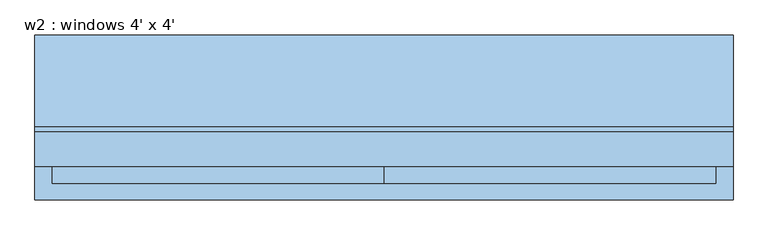
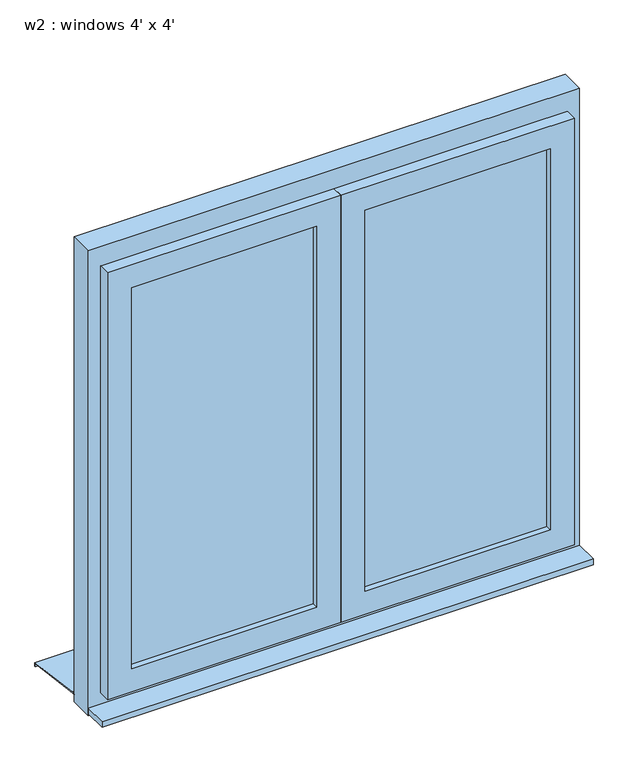
"""IFC4 building model written with IfcOpenShell, lengths in millimetres: window geometry, w2 : windows 4' x 4'."""

from ifc_helpers import new_model, si_unit, frame, origin, place, context, project, spatial, polyline, outline, extrude, faceted_brep, source, transform, mapped, element, save


def w2_windows_4_x_4_9dec5fc7(model_context):
    return source(origin(), model_context, "Body", "SolidModel", [
        extrude(outline(polyline([(-15.6778457, 1020.0), (144.3, 1000.0), (144.3, 990.0), (142.3, 990.0), (142.3, 998.3604634), (-15.8759277, 1018.0), (-25.7, 1018.0), (-25.7, 1020.0), (-15.6778457, 1020.0)])), frame((-609.6, 0.0, 0.0), z_axis=(1.0, 0.0, 0.0), x_axis=(0.0, 1.0, 0.0)), (0.0, 0.0, 1.0), 1219.2),
        extrude(outline(polyline([(-609.6, -144.3), (-609.6, -85.7), (609.6, -85.7), (609.6, -144.3), (-609.6, -144.3)])), frame((0.0, 0.0, 1005.0), z_axis=(0.0, 0.0, 1.0), x_axis=(1.0, 0.0, 0.0)), (0.0, 0.0, 1.0), 15.0),
        extrude(outline(polyline([(60.0, -70.7), (519.6, -70.7), (519.6, -100.7), (60.0, -100.7), (60.0, -70.7)])), frame((0.0, 0.0, 1110.0), z_axis=(0.0, 0.0, 1.0), x_axis=(1.0, 0.0, 0.0)), (0.0, 0.0, 1.0), 999.2),
        extrude(outline(polyline([(-519.6, -70.7), (-60.0, -70.7), (-60.0, -100.7), (-519.6, -100.7), (-519.6, -70.7)])), frame((0.0, 0.0, 1110.0), z_axis=(0.0, 0.0, 1.0), x_axis=(1.0, 0.0, 0.0)), (0.0, 0.0, 1.0), 999.2),
        extrude(outline(polyline([(2219.2, -609.6), (1000.0, -609.6), (1000.0, 609.6), (2219.2, 609.6), (2219.2, -609.6)]), holes=[polyline([(2139.2, -549.6), (2139.2, 549.6), (1080.0, 549.6), (1080.0, -549.6), (2139.2, -549.6)])]), frame((0.0, -85.7, 0.0), z_axis=(0.0, 1.0, 0.0), x_axis=(0.0, 0.0, 1.0)), (0.0, 0.0, 1.0), 60.0),
        extrude(outline(polyline([(30.0, -85.7), (-30.0, -85.7), (-30.0, -25.7), (30.0, -25.7), (30.0, -85.7)])), frame((0.0, 0.0, 1080.0), z_axis=(0.0, 0.0, 1.0), x_axis=(1.0, 0.0, 0.0)), (0.0, 0.0, 1.0), 1059.2),
        faceted_brep([(30.0, -85.7, 1080.0), (30.0, -55.7, 1080.0), (549.6, -55.7, 1080.0), (549.6, -85.7, 1080.0), (549.6, -55.7, 2139.2), (549.6, -85.7, 2139.2), (30.0, -55.7, 2139.2), (519.6, -55.7, 2109.2), (60.0, -55.7, 2109.2), (60.0, -55.7, 1110.0), (519.6, -55.7, 1110.0), (579.6, -85.7, 1050.0), (0.0, -85.7, 1050.0), (0.0, -85.7, 2169.2), (579.6, -85.7, 2169.2), (30.0, -85.7, 2139.2), (0.0, -115.7, 1050.0), (579.6, -115.7, 1050.0), (579.6, -115.7, 2169.2), (0.0, -115.7, 2169.2), (519.6, -115.7, 1110.0), (60.0, -115.7, 1110.0), (60.0, -115.7, 2109.2), (519.6, -115.7, 2109.2)], [[[0, 1, 2, 3]], [[3, 2, 4, 5]], [[2, 1, 6, 4], [7, 8, 9, 10]], [[11, 12, 13, 14], [5, 15, 0, 3]], [[16, 12, 11, 17]], [[17, 11, 14, 18]], [[18, 19, 16, 17], [20, 21, 22, 23]], [[9, 21, 20, 10]], [[10, 20, 23, 7]], [[15, 6, 1, 0]], [[19, 13, 12, 16]], [[8, 22, 21, 9]], [[5, 4, 6, 15]], [[18, 14, 13, 19]], [[7, 23, 22, 8]]]),
        faceted_brep([(-549.6, -85.7, 1080.0), (-549.6, -55.7, 1080.0), (-30.0, -55.7, 1080.0), (-30.0, -85.7, 1080.0), (-30.0, -55.7, 2139.2), (-30.0, -85.7, 2139.2), (-549.6, -55.7, 2139.2), (-60.0, -55.7, 2109.2), (-519.6, -55.7, 2109.2), (-519.6, -55.7, 1110.0), (-60.0, -55.7, 1110.0), (0.0, -85.7, 1050.0), (-579.6, -85.7, 1050.0), (-579.6, -85.7, 2169.2), (0.0, -85.7, 2169.2), (-549.6, -85.7, 2139.2), (-579.6, -115.7, 1050.0), (0.0, -115.7, 1050.0), (0.0, -115.7, 2169.2), (-579.6, -115.7, 2169.2), (-60.0, -115.7, 1110.0), (-519.6, -115.7, 1110.0), (-519.6, -115.7, 2109.2), (-60.0, -115.7, 2109.2)], [[[0, 1, 2, 3]], [[3, 2, 4, 5]], [[2, 1, 6, 4], [7, 8, 9, 10]], [[11, 12, 13, 14], [5, 15, 0, 3]], [[16, 12, 11, 17]], [[17, 11, 14, 18]], [[18, 19, 16, 17], [20, 21, 22, 23]], [[9, 21, 20, 10]], [[10, 20, 23, 7]], [[15, 6, 1, 0]], [[19, 13, 12, 16]], [[8, 22, 21, 9]], [[5, 4, 6, 15]], [[18, 14, 13, 19]], [[7, 23, 22, 8]]]),
    ])


if __name__ == "__main__":
    model = new_model("IFC4")
    model_context = context("Model", 3, world=origin())
    ifc_project = project(units=[si_unit("LENGTHUNIT", "METRE", prefix="MILLI")], contexts=[model_context])
    site = spatial("IfcSite", under=ifc_project)
    building = spatial("IfcBuilding", under=site)
    placement = place(None, origin())
    w2_windows_4_x_4_shape = w2_windows_4_x_4_9dec5fc7(model_context)
    element("IfcWindow", 1, ObjectType="w2 : windows 4' x 4'", at=placement, inside=building, context=model_context, shape_type="MappedRepresentation", body=[
        mapped(w2_windows_4_x_4_shape, transform((0.0, 0.0, 0.0), x_axis=(1.0, 0.0, 0.0), y_axis=(0.0, 1.0, 0.0), z_axis=(0.0, 0.0, 1.0))),
    ])
    save(model, "model.ifc")

# Revit data of these elements
# Type "w2 : windows 4' x 4'"
#   Type Mark = "31"
#   Operation = "DoublePanelVertical"
#   Keynote = "16.05.01"
#   Analytic Construction = "<None>"
#   Rough Width = 4' - 0"
#   Rough Height = 4' - 0"
#   Rahmentiefe = 0' - 2.3622"
#   Rahmenhöhe unten = 0' - 3.14961"
#   Rahmehöhe oben = 0' - 3.14961"
#   Rahmenbreite = 0' - 2.3622"
#   Heat Transfer Coefficient (U) = 2.81836 BTU/(h·ft²·°F)
#   Height = 4' - 0"
#   Flügeltiefe = 0' - 2.3622"
#   Flügelbreite = 0' - 2.3622"
#   Einbautiefe (von außen) [instance default] = 0' - 5.51181"
#   Width = 4' - 0"
#   Kippflügel [instance default] = yes
#   Drehflügel im Grundriß darstellen [instance default] = no
#   Drehflügel [instance default] = yes
#   Define Thermal Properties by = 1
#   Rahmen [instance default] = none
#   Glas [instance default] = blue glass
#   Flügel [instance default] = WINDOW COLOUR WHITE
#   Fensterbank aussen [instance default] = WINDOW COLOUR WHITE
#   Fensterbank innen [instance default] = WINDOW COLOUR WHITE
#   Visual Light Transmittance = 0
#   Thermal Resistance (R) = 0
#   Solar Heat Gain Coefficient = 0
#   Wall Closure = (empty or 0)
# Element 1 (IfcWindow, "w2 : windows 4' x 4'")
#   Materials on its faces: "WINDOW COLOUR WHITE", "blue glass"
# Materials
#   "blue glass": class "System", colour RGB 0 0 255, transparency 0.75, Cost = 0
#   "WINDOW COLOUR WHITE": class "Generic", colour RGB 120 120 120, transparency 0, Cost = 0
